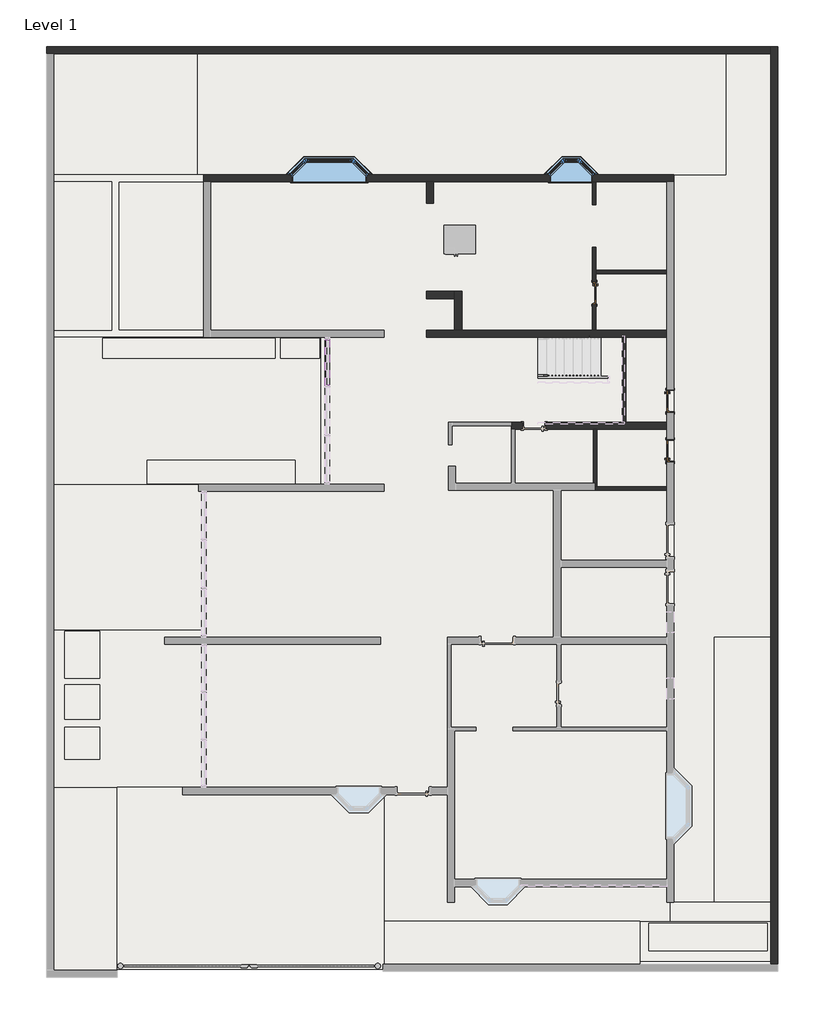
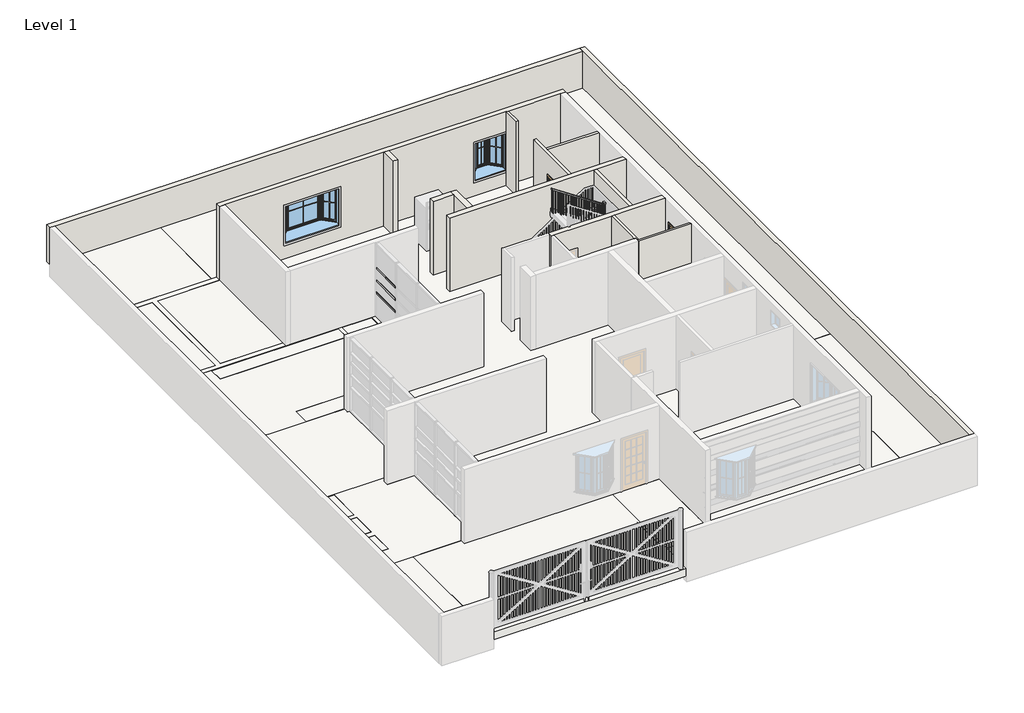
# One storey, part 4 of 5: 15 slabs, 14 walls, 3 doors, 3 members, 2 windows, 1 railing.
"""IFC4 building model written with IfcOpenShell, lengths in millimetres."""

from ifc_helpers import new_model, si_unit, frame, origin, origin_with_axes, place, context, project, spatial, polyline, outline, extrude, faceted_brep, transform, mapped, element, save
from components import door_interior_single_1_panel_wood_5fe0af8f, door_interior_single_1_panel_wood_a1a047a4, door_interior_single_1_panel_wood_33af59b7, member_f9f7e124, window_9f89e8e4, window_bay_casement_45_degree_angle_window_4_787d36ed

model = new_model("IFC4")

# Units and contexts
model_context = context("Model", 3, world=origin())
ifc_project = project(units=[si_unit("LENGTHUNIT", "METRE", prefix="MILLI")], contexts=[model_context])

# Site, building, storey
site = spatial("IfcSite", under=ifc_project)
building = spatial("IfcBuilding", under=site)
storey = spatial("IfcBuildingStorey", under=building, Name="Level 1", Elevation=0.0)

# Doors
placement = place(None, origin())
door_interior_single_1_panel_wood_shape = door_interior_single_1_panel_wood_5fe0af8f(model_context)
element("IfcDoor", 1, ObjectType="Door-Interior-Single-1_Panel-Wood", at=placement, inside=storey, context=model_context, shape_type="MappedRepresentation", body=[
    mapped(door_interior_single_1_panel_wood_shape, transform((-37351.3130314, 2521.1086027, 0.0), x_axis=(0.0, 1.0, 0.0), y_axis=(-1.0, 0.0, 0.0), z_axis=(0.0, 0.0, 1.0))),
])
door_interior_single_1_panel_wood_2_shape = door_interior_single_1_panel_wood_a1a047a4(model_context)
element("IfcDoor", 2, ObjectType="Door-Interior-Single-1_Panel-Wood", at=placement, inside=storey, context=model_context, shape_type="MappedRepresentation", body=[
    mapped(door_interior_single_1_panel_wood_2_shape, transform((-37351.3130314, 3943.5086027, 0.0), x_axis=(0.0, -1.0, 0.0), y_axis=(1.0, 0.0, 0.0), z_axis=(0.0, 0.0, 1.0))),
])
door_interior_single_1_panel_wood_3_shape = door_interior_single_1_panel_wood_33af59b7(model_context)
element("IfcDoor", 3, ObjectType="Door-Interior-Single-1_Panel-Wood", at=placement, inside=storey, context=model_context, shape_type="MappedRepresentation", body=[
    mapped(door_interior_single_1_panel_wood_3_shape, transform((-39529.3630314, 7042.3086027, 0.0), x_axis=(0.0, -1.0, 0.0), y_axis=(1.0, 0.0, 0.0), z_axis=(0.0, 0.0, 1.0))),
])

# Members
member_shape = member_f9f7e124(model_context)
element("IfcMember", 4, ObjectType="Rectangular Mullion : 2.5\" x 5\" rectangular", at=placement, inside=storey, context=model_context, shape_type="MappedRepresentation", body=[
    mapped(member_shape, transform((-47203.3380314, 5708.8086027, 1016.0), x_axis=(0.0, 0.0, 1.0), y_axis=(1.0, 0.0, 0.0), z_axis=(0.0, 1.0, 0.0))),
])
element("IfcMember", 5, ObjectType="Rectangular Mullion : 2.5\" x 5\" rectangular", at=placement, inside=storey, context=model_context, shape_type="MappedRepresentation", body=[
    mapped(member_shape, transform((-47203.3380314, 5708.8086027, 2032.0), x_axis=(0.0, 0.0, 1.0), y_axis=(1.0, 0.0, 0.0), z_axis=(0.0, 1.0, 0.0))),
])
element("IfcMember", 6, ObjectType="Rectangular Mullion : 2.5\" x 5\" rectangular", at=placement, inside=storey, context=model_context, shape_type="MappedRepresentation", body=[
    mapped(member_shape, transform((-47203.3380314, 5708.8086027, 1524.0), x_axis=(0.0, 0.0, 1.0), y_axis=(1.0, 0.0, 0.0), z_axis=(0.0, 1.0, 0.0))),
])

# Railing
element("IfcRailing", 7, ObjectType="Handrail - Rectangular", at=placement, inside=storey, context=model_context, shape_type="SolidModel", body=[
    faceted_brep([(-41148.2472477, 4705.5086027, 1083.7333333), (-41148.2472477, 4705.5086027, 1022.6793317), (-41148.2472477, 4654.7086027, 1022.6793317), (-41148.2472477, 4654.7086027, 1083.7333333), (-39167.0472477, 4705.5086027, 2404.5333333), (-39116.2472477, 4705.5086027, 2377.3459984), (-39116.2472477, 4654.7086027, 2377.3459984), (-39167.0472477, 4654.7086027, 2404.5333333), (-39167.0472477, 4705.5086027, 2438.4), (-39116.2472477, 4705.5086027, 2387.6), (-39116.2472477, 4654.7086027, 2387.6), (-39167.0472477, 4654.7086027, 2438.4), (-39040.0472477, 4705.5086027, 2438.4), (-39040.0472477, 4705.5086027, 2387.6), (-39090.8472477, 4654.7086027, 2387.6), (-39090.8472477, 4654.7086027, 2438.4), (-39040.0472477, 4578.5086027, 2438.4), (-39040.0472477, 4578.5086027, 2387.6), (-39090.8472477, 4578.5086027, 2387.6), (-39090.8472477, 4578.5086027, 2438.4), (-39040.0472477, 4527.7086027, 2438.4), (-39040.0472477, 4476.9086027, 2387.6), (-39090.8472477, 4476.9086027, 2387.6), (-39090.8472477, 4527.7086027, 2438.4), (-39040.0472477, 4527.7086027, 2641.6), (-39040.0472477, 4476.9086027, 2590.8), (-39090.8472477, 4476.9086027, 2590.8), (-39090.8472477, 4527.7086027, 2641.6), (-39040.0472477, 4400.7086027, 2641.6), (-39040.0472477, 4400.7086027, 2590.8), (-39090.8472477, 4451.5086027, 2590.8), (-39090.8472477, 4451.5086027, 2641.6), (-39167.0472477, 4400.7086027, 2641.6), (-39182.4282501, 4400.7086027, 2590.8), (-39182.4282501, 4451.5086027, 2590.8), (-39167.0472477, 4451.5086027, 2641.6), (-41148.2472477, 4400.7086027, 3962.4), (-41148.2472477, 4451.5086027, 3962.4), (-41148.2472477, 4451.5086027, 3901.3459984), (-41148.2472477, 4400.7086027, 3901.3459984)], [[[0, 1, 2, 3]], [[1, 0, 4, 5]], [[2, 1, 5, 6]], [[3, 2, 6, 7]], [[0, 3, 7, 4]], [[5, 4, 8, 9]], [[6, 5, 9, 10]], [[7, 6, 10, 11]], [[4, 7, 11, 8]], [[9, 8, 12, 13]], [[10, 9, 13, 14]], [[11, 10, 14, 15]], [[8, 11, 15, 12]], [[13, 12, 16, 17]], [[14, 13, 17, 18]], [[15, 14, 18, 19]], [[12, 15, 19, 16]], [[17, 16, 20, 21]], [[18, 17, 21, 22]], [[19, 18, 22, 23]], [[16, 19, 23, 20]], [[21, 20, 24, 25]], [[22, 21, 25, 26]], [[23, 22, 26, 27]], [[20, 23, 27, 24]], [[25, 24, 28, 29]], [[26, 25, 29, 30]], [[27, 26, 30, 31]], [[24, 27, 31, 28]], [[29, 28, 32, 33]], [[30, 29, 33, 34]], [[31, 30, 34, 35]], [[28, 31, 35, 32]], [[36, 37, 38, 39]], [[33, 32, 36, 39]], [[34, 33, 39, 38]], [[35, 34, 38, 37]], [[32, 35, 37, 36]]]),
    extrude(outline(polyline([(3861.1293317, -41087.9222477), (3873.8293317, -41106.9722477), (2878.6666667, -41106.9722477), (2878.6666667, -41087.9222477), (3861.1293317, -41087.9222477)])), frame((0.0, 4416.5836027, 0.0), z_axis=(0.0, 1.0, 0.0), x_axis=(0.0, 0.0, 1.0)), (0.0, 0.0, 1.0), 19.05),
    extrude(outline(polyline([(3793.3959984, -40986.3222477), (3806.0959984, -41005.3722477), (2878.6666667, -41005.3722477), (2878.6666667, -40986.3222477), (3793.3959984, -40986.3222477)])), frame((0.0, 4416.5836027, 0.0), z_axis=(0.0, 1.0, 0.0), x_axis=(0.0, 0.0, 1.0)), (0.0, 0.0, 1.0), 19.05),
    extrude(outline(polyline([(3725.6626651, -40884.7222477), (3738.3626651, -40903.7722477), (2878.6666667, -40903.7722477), (2878.6666667, -40884.7222477), (3725.6626651, -40884.7222477)])), frame((0.0, 4416.5836027, 0.0), z_axis=(0.0, 1.0, 0.0), x_axis=(0.0, 0.0, 1.0)), (0.0, 0.0, 1.0), 19.05),
    extrude(outline(polyline([(3657.9293317, -40783.1222477), (3670.6293317, -40802.1722477), (2709.3333333, -40802.1722477), (2709.3333333, -40783.1222477), (3657.9293317, -40783.1222477)])), frame((0.0, 4416.5836027, 0.0), z_axis=(0.0, 1.0, 0.0), x_axis=(0.0, 0.0, 1.0)), (0.0, 0.0, 1.0), 19.05),
    extrude(outline(polyline([(3590.1959984, -40681.5222477), (3602.8959984, -40700.5722477), (2709.3333333, -40700.5722477), (2709.3333333, -40681.5222477), (3590.1959984, -40681.5222477)])), frame((0.0, 4416.5836027, 0.0), z_axis=(0.0, 1.0, 0.0), x_axis=(0.0, 0.0, 1.0)), (0.0, 0.0, 1.0), 19.05),
    extrude(outline(polyline([(3522.4626651, -40579.9222477), (3535.1626651, -40598.9722477), (2540.0, -40598.9722477), (2540.0, -40579.9222477), (3522.4626651, -40579.9222477)])), frame((0.0, 4416.5836027, 0.0), z_axis=(0.0, 1.0, 0.0), x_axis=(0.0, 0.0, 1.0)), (0.0, 0.0, 1.0), 19.05),
    extrude(outline(polyline([(3454.7293317, -40478.3222477), (3467.4293317, -40497.3722477), (2540.0, -40497.3722477), (2540.0, -40478.3222477), (3454.7293317, -40478.3222477)])), frame((0.0, 4416.5836027, 0.0), z_axis=(0.0, 1.0, 0.0), x_axis=(0.0, 0.0, 1.0)), (0.0, 0.0, 1.0), 19.05),
    extrude(outline(polyline([(3386.9959984, -40376.7222477), (3399.6959984, -40395.7722477), (2540.0, -40395.7722477), (2540.0, -40376.7222477), (3386.9959984, -40376.7222477)])), frame((0.0, 4416.5836027, 0.0), z_axis=(0.0, 1.0, 0.0), x_axis=(0.0, 0.0, 1.0)), (0.0, 0.0, 1.0), 19.05),
    extrude(outline(polyline([(3319.2626651, -40275.1222477), (3331.9626651, -40294.1722477), (2370.6666667, -40294.1722477), (2370.6666667, -40275.1222477), (3319.2626651, -40275.1222477)])), frame((0.0, 4416.5836027, 0.0), z_axis=(0.0, 1.0, 0.0), x_axis=(0.0, 0.0, 1.0)), (0.0, 0.0, 1.0), 19.05),
    extrude(outline(polyline([(3251.5293317, -40173.5222477), (3264.2293317, -40192.5722477), (2370.6666667, -40192.5722477), (2370.6666667, -40173.5222477), (3251.5293317, -40173.5222477)])), frame((0.0, 4416.5836027, 0.0), z_axis=(0.0, 1.0, 0.0), x_axis=(0.0, 0.0, 1.0)), (0.0, 0.0, 1.0), 19.05),
    extrude(outline(polyline([(3183.7959984, -40071.9222477), (3196.4959984, -40090.9722477), (2201.3333333, -40090.9722477), (2201.3333333, -40071.9222477), (3183.7959984, -40071.9222477)])), frame((0.0, 4416.5836027, 0.0), z_axis=(0.0, 1.0, 0.0), x_axis=(0.0, 0.0, 1.0)), (0.0, 0.0, 1.0), 19.05),
    extrude(outline(polyline([(3116.0626651, -39970.3222477), (3128.7626651, -39989.3722477), (2201.3333333, -39989.3722477), (2201.3333333, -39970.3222477), (3116.0626651, -39970.3222477)])), frame((0.0, 4416.5836027, 0.0), z_axis=(0.0, 1.0, 0.0), x_axis=(0.0, 0.0, 1.0)), (0.0, 0.0, 1.0), 19.05),
    extrude(outline(polyline([(3048.3293317, -39868.7222477), (3061.0293317, -39887.7722477), (2201.3333333, -39887.7722477), (2201.3333333, -39868.7222477), (3048.3293317, -39868.7222477)])), frame((0.0, 4416.5836027, 0.0), z_axis=(0.0, 1.0, 0.0), x_axis=(0.0, 0.0, 1.0)), (0.0, 0.0, 1.0), 19.05),
    extrude(outline(polyline([(2980.5959984, -39767.1222477), (2993.2959984, -39786.1722477), (2032.0, -39786.1722477), (2032.0, -39767.1222477), (2980.5959984, -39767.1222477)])), frame((0.0, 4416.5836027, 0.0), z_axis=(0.0, 1.0, 0.0), x_axis=(0.0, 0.0, 1.0)), (0.0, 0.0, 1.0), 19.05),
    extrude(outline(polyline([(2912.8626651, -39665.5222477), (2925.5626651, -39684.5722477), (2032.0, -39684.5722477), (2032.0, -39665.5222477), (2912.8626651, -39665.5222477)])), frame((0.0, 4416.5836027, 0.0), z_axis=(0.0, 1.0, 0.0), x_axis=(0.0, 0.0, 1.0)), (0.0, 0.0, 1.0), 19.05),
    extrude(outline(polyline([(2845.1293317, -39563.9222477), (2857.8293317, -39582.9722477), (1862.6666667, -39582.9722477), (1862.6666667, -39563.9222477), (2845.1293317, -39563.9222477)])), frame((0.0, 4416.5836027, 0.0), z_axis=(0.0, 1.0, 0.0), x_axis=(0.0, 0.0, 1.0)), (0.0, 0.0, 1.0), 19.05),
    extrude(outline(polyline([(2777.3959984, -39462.3222477), (2790.0959984, -39481.3722477), (1862.6666667, -39481.3722477), (1862.6666667, -39462.3222477), (2777.3959984, -39462.3222477)])), frame((0.0, 4416.5836027, 0.0), z_axis=(0.0, 1.0, 0.0), x_axis=(0.0, 0.0, 1.0)), (0.0, 0.0, 1.0), 19.05),
    extrude(outline(polyline([(2709.6626651, -39360.7222477), (2722.3626651, -39379.7722477), (1862.6666667, -39379.7722477), (1862.6666667, -39360.7222477), (2709.6626651, -39360.7222477)])), frame((0.0, 4416.5836027, 0.0), z_axis=(0.0, 1.0, 0.0), x_axis=(0.0, 0.0, 1.0)), (0.0, 0.0, 1.0), 19.05),
    extrude(outline(polyline([(2641.9293317, -39259.1222477), (2654.6293317, -39278.1722477), (1693.3333333, -39278.1722477), (1693.3333333, -39259.1222477), (2641.9293317, -39259.1222477)])), frame((0.0, 4416.5836027, 0.0), z_axis=(0.0, 1.0, 0.0), x_axis=(0.0, 0.0, 1.0)), (0.0, 0.0, 1.0), 19.05),
    extrude(outline(polyline([(2574.1959984, -39157.5222477), (2586.8959984, -39176.5722477), (1693.3333333, -39176.5722477), (1693.3333333, -39157.5222477), (2574.1959984, -39157.5222477)])), frame((0.0, 4416.5836027, 0.0), z_axis=(0.0, 1.0, 0.0), x_axis=(0.0, 0.0, 1.0)), (0.0, 0.0, 1.0), 19.05),
    extrude(outline(polyline([(-39074.9722477, 4486.4336027), (-39055.9222477, 4486.4336027), (-39055.9222477, 4467.3836027), (-39074.9722477, 4467.3836027), (-39074.9722477, 4486.4336027)])), frame((0.0, 0.0, 1524.0), z_axis=(0.0, 0.0, 1.0), x_axis=(1.0, 0.0, 0.0)), (0.0, 0.0, 1.0), 1066.8),
    extrude(outline(polyline([(-39074.9722477, 4588.0336027), (-39055.9222477, 4588.0336027), (-39055.9222477, 4568.9836027), (-39074.9722477, 4568.9836027), (-39074.9722477, 4588.0336027)])), frame((0.0, 0.0, 1524.0), z_axis=(0.0, 0.0, 1.0), x_axis=(1.0, 0.0, 0.0)), (0.0, 0.0, 1.0), 863.6),
    extrude(outline(polyline([(-39125.7722477, 4670.5836027), (-39125.7722477, 4689.6336027), (-39106.7222477, 4689.6336027), (-39106.7222477, 4670.5836027), (-39125.7722477, 4670.5836027)])), frame((0.0, 0.0, 1524.0), z_axis=(0.0, 0.0, 1.0), x_axis=(1.0, 0.0, 0.0)), (0.0, 0.0, 1.0), 863.6),
    extrude(outline(polyline([(2315.9626651, -39208.3222477), (2303.2626651, -39227.3722477), (1354.6666667, -39227.3722477), (1354.6666667, -39208.3222477), (2315.9626651, -39208.3222477)])), frame((0.0, 4670.5836027, 0.0), z_axis=(0.0, 1.0, 0.0), x_axis=(0.0, 0.0, 1.0)), (0.0, 0.0, 1.0), 19.05),
    extrude(outline(polyline([(2248.2293317, -39309.9222477), (2235.5293317, -39328.9722477), (1354.6666667, -39328.9722477), (1354.6666667, -39309.9222477), (2248.2293317, -39309.9222477)])), frame((0.0, 4670.5836027, 0.0), z_axis=(0.0, 1.0, 0.0), x_axis=(0.0, 0.0, 1.0)), (0.0, 0.0, 1.0), 19.05),
    extrude(outline(polyline([(2180.4959984, -39411.5222477), (2167.7959984, -39430.5722477), (1185.3333333, -39430.5722477), (1185.3333333, -39411.5222477), (2180.4959984, -39411.5222477)])), frame((0.0, 4670.5836027, 0.0), z_axis=(0.0, 1.0, 0.0), x_axis=(0.0, 0.0, 1.0)), (0.0, 0.0, 1.0), 19.05),
    extrude(outline(polyline([(2112.7626651, -39513.1222477), (2100.0626651, -39532.1722477), (1185.3333333, -39532.1722477), (1185.3333333, -39513.1222477), (2112.7626651, -39513.1222477)])), frame((0.0, 4670.5836027, 0.0), z_axis=(0.0, 1.0, 0.0), x_axis=(0.0, 0.0, 1.0)), (0.0, 0.0, 1.0), 19.05),
    extrude(outline(polyline([(2045.0293317, -39614.7222477), (2032.3293317, -39633.7722477), (1185.3333333, -39633.7722477), (1185.3333333, -39614.7222477), (2045.0293317, -39614.7222477)])), frame((0.0, 4670.5836027, 0.0), z_axis=(0.0, 1.0, 0.0), x_axis=(0.0, 0.0, 1.0)), (0.0, 0.0, 1.0), 19.05),
    extrude(outline(polyline([(1977.2959984, -39716.3222477), (1964.5959984, -39735.3722477), (1016.0, -39735.3722477), (1016.0, -39716.3222477), (1977.2959984, -39716.3222477)])), frame((0.0, 4670.5836027, 0.0), z_axis=(0.0, 1.0, 0.0), x_axis=(0.0, 0.0, 1.0)), (0.0, 0.0, 1.0), 19.05),
    extrude(outline(polyline([(1909.5626651, -39817.9222477), (1896.8626651, -39836.9722477), (1016.0, -39836.9722477), (1016.0, -39817.9222477), (1909.5626651, -39817.9222477)])), frame((0.0, 4670.5836027, 0.0), z_axis=(0.0, 1.0, 0.0), x_axis=(0.0, 0.0, 1.0)), (0.0, 0.0, 1.0), 19.05),
    extrude(outline(polyline([(1841.8293317, -39919.5222477), (1829.1293317, -39938.5722477), (846.6666667, -39938.5722477), (846.6666667, -39919.5222477), (1841.8293317, -39919.5222477)])), frame((0.0, 4670.5836027, 0.0), z_axis=(0.0, 1.0, 0.0), x_axis=(0.0, 0.0, 1.0)), (0.0, 0.0, 1.0), 19.05),
    extrude(outline(polyline([(1774.0959984, -40021.1222477), (1761.3959984, -40040.1722477), (846.6666667, -40040.1722477), (846.6666667, -40021.1222477), (1774.0959984, -40021.1222477)])), frame((0.0, 4670.5836027, 0.0), z_axis=(0.0, 1.0, 0.0), x_axis=(0.0, 0.0, 1.0)), (0.0, 0.0, 1.0), 19.05),
    extrude(outline(polyline([(1706.3626651, -40122.7222477), (1693.6626651, -40141.7722477), (846.6666667, -40141.7722477), (846.6666667, -40122.7222477), (1706.3626651, -40122.7222477)])), frame((0.0, 4670.5836027, 0.0), z_axis=(0.0, 1.0, 0.0), x_axis=(0.0, 0.0, 1.0)), (0.0, 0.0, 1.0), 19.05),
    extrude(outline(polyline([(1638.6293317, -40224.3222477), (1625.9293317, -40243.3722477), (677.3333333, -40243.3722477), (677.3333333, -40224.3222477), (1638.6293317, -40224.3222477)])), frame((0.0, 4670.5836027, 0.0), z_axis=(0.0, 1.0, 0.0), x_axis=(0.0, 0.0, 1.0)), (0.0, 0.0, 1.0), 19.05),
    extrude(outline(polyline([(1570.8959984, -40325.9222477), (1558.1959984, -40344.9722477), (677.3333333, -40344.9722477), (677.3333333, -40325.9222477), (1570.8959984, -40325.9222477)])), frame((0.0, 4670.5836027, 0.0), z_axis=(0.0, 1.0, 0.0), x_axis=(0.0, 0.0, 1.0)), (0.0, 0.0, 1.0), 19.05),
    extrude(outline(polyline([(1503.1626651, -40427.5222477), (1490.4626651, -40446.5722477), (508.0, -40446.5722477), (508.0, -40427.5222477), (1503.1626651, -40427.5222477)])), frame((0.0, 4670.5836027, 0.0), z_axis=(0.0, 1.0, 0.0), x_axis=(0.0, 0.0, 1.0)), (0.0, 0.0, 1.0), 19.05),
    extrude(outline(polyline([(1435.4293317, -40529.1222477), (1422.7293317, -40548.1722477), (508.0, -40548.1722477), (508.0, -40529.1222477), (1435.4293317, -40529.1222477)])), frame((0.0, 4670.5836027, 0.0), z_axis=(0.0, 1.0, 0.0), x_axis=(0.0, 0.0, 1.0)), (0.0, 0.0, 1.0), 19.05),
    extrude(outline(polyline([(1367.6959984, -40630.7222477), (1354.9959984, -40649.7722477), (508.0, -40649.7722477), (508.0, -40630.7222477), (1367.6959984, -40630.7222477)])), frame((0.0, 4670.5836027, 0.0), z_axis=(0.0, 1.0, 0.0), x_axis=(0.0, 0.0, 1.0)), (0.0, 0.0, 1.0), 19.05),
    extrude(outline(polyline([(1299.9626651, -40732.3222477), (1287.2626651, -40751.3722477), (338.6666667, -40751.3722477), (338.6666667, -40732.3222477), (1299.9626651, -40732.3222477)])), frame((0.0, 4670.5836027, 0.0), z_axis=(0.0, 1.0, 0.0), x_axis=(0.0, 0.0, 1.0)), (0.0, 0.0, 1.0), 19.05),
    extrude(outline(polyline([(1232.2293317, -40833.9222477), (1219.5293317, -40852.9722477), (338.6666667, -40852.9722477), (338.6666667, -40833.9222477), (1232.2293317, -40833.9222477)])), frame((0.0, 4670.5836027, 0.0), z_axis=(0.0, 1.0, 0.0), x_axis=(0.0, 0.0, 1.0)), (0.0, 0.0, 1.0), 19.05),
    extrude(outline(polyline([(1164.4959984, -40935.5222477), (1151.7959984, -40954.5722477), (169.3333333, -40954.5722477), (169.3333333, -40935.5222477), (1164.4959984, -40935.5222477)])), frame((0.0, 4670.5836027, 0.0), z_axis=(0.0, 1.0, 0.0), x_axis=(0.0, 0.0, 1.0)), (0.0, 0.0, 1.0), 19.05),
    extrude(outline(polyline([(1096.7626651, -41037.1222477), (1084.0626651, -41056.1722477), (169.3333333, -41056.1722477), (169.3333333, -41037.1222477), (1096.7626651, -41037.1222477)])), frame((0.0, 4670.5836027, 0.0), z_axis=(0.0, 1.0, 0.0), x_axis=(0.0, 0.0, 1.0)), (0.0, 0.0, 1.0), 19.05),
    extrude(outline(polyline([(-39074.9722477, 4435.6336027), (-39055.9222477, 4435.6336027), (-39055.9222477, 4416.5836027), (-39074.9722477, 4416.5836027), (-39074.9722477, 4435.6336027)])), frame((0.0, 0.0, 1524.0), z_axis=(0.0, 0.0, 1.0), x_axis=(1.0, 0.0, 0.0)), (0.0, 0.0, 1.0), 1066.8),
    extrude(outline(polyline([(-39074.9722477, 4670.5836027), (-39074.9722477, 4689.6336027), (-39055.9222477, 4689.6336027), (-39055.9222477, 4670.5836027), (-39074.9722477, 4670.5836027)])), frame((0.0, 0.0, 1524.0), z_axis=(0.0, 0.0, 1.0), x_axis=(1.0, 0.0, 0.0)), (0.0, 0.0, 1.0), 863.6),
    extrude(outline(polyline([(3888.6459984, -41129.1972477), (3901.3459984, -41148.2472477), (2878.6666667, -41148.2472477), (2878.6666667, -41129.1972477), (3888.6459984, -41129.1972477)])), frame((0.0, 4416.5836027, 0.0), z_axis=(0.0, 1.0, 0.0), x_axis=(0.0, 0.0, 1.0)), (0.0, 0.0, 1.0), 19.05),
    extrude(outline(polyline([(1035.3793317, -41129.1972477), (1022.6793317, -41148.2472477), (169.3333333, -41148.2472477), (169.3333333, -41129.1972477), (1035.3793317, -41129.1972477)])), frame((0.0, 4670.5836027, 0.0), z_axis=(0.0, 1.0, 0.0), x_axis=(0.0, 0.0, 1.0)), (0.0, 0.0, 1.0), 19.05),
])

# Slabs
element("IfcSlab", 8, at=placement, inside=storey, context=model_context, shape_type="SweptSolid", body=[
    extrude(outline(polyline([(-50956.4260686, 13968.3227856), (-50956.4260686, 10445.9086027), (-55177.8412112, 10445.9086027), (-55177.8412112, 13968.3227856), (-50956.4260686, 13968.3227856)])), frame((0.0, 0.0, -304.8), z_axis=(0.0, 0.0, 1.0), x_axis=(1.0, 0.0, 0.0)), (0.0, 0.0, 1.0), 304.8),
    extrude(outline(polyline([(-38223.6402545, -12148.7888585), (-38223.6402545, -11006.389557), (-34350.9380314, -11006.389557), (-34350.9380314, -12148.7888585), (-38223.6402545, -12148.7888585)]), holes=[polyline([(-37969.6402545, -11843.9888585), (-34554.1380314, -11843.9888585), (-34554.1380314, -11057.189557), (-37969.6402545, -11057.189557), (-37969.6402545, -11843.9888585)])]), frame((0.0, 0.0, -304.8), z_axis=(0.0, 0.0, 1.0), x_axis=(1.0, 0.0, 0.0)), (0.0, 0.0, 1.0), 304.8),
])
element("IfcSlab", 9, at=placement, inside=storey, context=model_context, shape_type="SweptSolid", body=[
    extrude(outline(polyline([(-34350.9380314, -2838.2913973), (-34350.9380314, -10458.2913973), (-36081.491084, -10458.2913973), (-36081.491084, -2838.2913973), (-34350.9380314, -2838.2913973)])), frame((0.0, 0.0, -304.8), z_axis=(0.0, 0.0, 1.0), x_axis=(1.0, 0.0, 0.0)), (0.0, 0.0, 1.0), 304.8),
])
element("IfcSlab", 10, at=placement, inside=storey, context=model_context, shape_type="SweptSolid", body=[
    extrude(outline(polyline([(-55177.8412112, 10445.9086027), (-50759.3380314, 10445.9086027), (-50759.3380314, 10242.7086027), (-53197.7380314, 10242.7086027), (-53197.7380314, 5975.5086027), (-50759.3380314, 5975.5086027), (-50759.3380314, 5772.3086027), (-55204.3380314, 5772.3086027), (-55204.3380314, 5975.5086027), (-53400.9380314, 5975.5086027), (-53400.9380314, 10242.7086027), (-55204.3380314, 10242.7086027), (-55204.3380314, 10445.9086027), (-55177.8412112, 10445.9086027)])), frame((0.0, 0.0, -304.8), z_axis=(0.0, 0.0, 1.0), x_axis=(1.0, 0.0, 0.0)), (0.0, 0.0, 1.0), 304.8),
])
element("IfcSlab", 11, ObjectType="GRASS TYPE 1'", at=placement, inside=storey, context=model_context, shape_type="SweptSolid", body=[
    extrude(outline(polyline([(-55204.3380314, -2635.0913973), (-50759.3380314, -2635.0913973), (-50759.3380314, -7156.2913973), (-55204.3380314, -7156.2913973), (-55204.3380314, -2635.0913973)]), holes=[polyline([(-53746.793915, -4017.7088102), (-53746.793915, -2671.5088102), (-54750.550784, -2671.5088102), (-54750.550784, -4017.7088102), (-53746.793915, -4017.7088102)]), polyline([(-54750.550784, -4205.0162107), (-54750.550784, -5196.8737449), (-53746.793915, -5196.8737449), (-53746.793915, -4205.0162107), (-54750.550784, -4205.0162107)]), polyline([(-54750.550784, -5426.5355358), (-54750.550784, -6340.9585066), (-53746.793915, -6340.9585066), (-53746.793915, -5426.5355358), (-54750.550784, -5426.5355358)])]), frame((0.0, 0.0, -304.8), z_axis=(0.0, 0.0, 1.0), x_axis=(1.0, 0.0, 0.0)), (0.0, 0.0, 1.0), 304.8),
])
element("IfcSlab", 12, ObjectType="GRASS TYPE 1'", at=placement, inside=storey, context=model_context, shape_type="SweptSolid", body=[
    extrude(outline(polyline([(-55204.3380314, 5772.3086027), (-47406.5380314, 5772.3086027), (-47406.5380314, 1555.9086027), (-55204.3380314, 1555.9086027), (-55204.3380314, 5772.3086027)]), holes=[polyline([(-48135.4981877, 2238.2630791), (-52386.7116594, 2238.2630791), (-52386.7116594, 1573.668759), (-48135.4981877, 1573.668759), (-48135.4981877, 2238.2630791)]), polyline([(-47424.2981877, 5180.468759), (-47424.2981877, 5754.5484465), (-48553.7407394, 5754.5484465), (-48553.7407394, 5180.468759), (-47424.2981877, 5180.468759)]), polyline([(-48713.9410385, 5180.468759), (-48713.9410385, 5754.5484465), (-53668.2114737, 5754.5484465), (-53668.2114737, 5180.468759), (-48713.9410385, 5180.468759)])]), frame((0.0, 0.0, -304.8), z_axis=(0.0, 0.0, 1.0), x_axis=(1.0, 0.0, 0.0)), (0.0, 0.0, 1.0), 304.8),
])
element("IfcSlab", 13, ObjectType="GRASS TYPE 1'", at=placement, inside=storey, context=model_context, shape_type="SweptSolid", body=[
    extrude(outline(polyline([(-55204.3380314, -7156.2913973), (-53248.5380314, -7156.2913973), (-53248.5380314, -12388.6913973), (-55204.3380314, -12388.6913973), (-55204.3380314, -7156.2913973)])), frame((0.0, 0.0, -304.8), z_axis=(0.0, 0.0, 1.0), x_axis=(1.0, 0.0, 0.0)), (0.0, 0.0, 1.0), 304.8),
    extrude(outline(polyline([(-45577.7380314, -11006.389557), (-38223.6402545, -11006.389557), (-38223.6402545, -12386.9889249), (-45577.7380314, -12386.9889249), (-45577.7380314, -11006.389557)])), frame((0.0, 0.0, -304.8), z_axis=(0.0, 0.0, 1.0), x_axis=(1.0, 0.0, 0.0)), (0.0, 0.0, 1.0), 304.8),
    extrude(outline(polyline([(-37969.6402545, -11057.189557), (-34554.1380314, -11057.189557), (-34554.1380314, -11843.9888585), (-37969.6402545, -11843.9888585), (-37969.6402545, -11057.189557)])), frame((0.0, 0.0, -304.8), z_axis=(0.0, 0.0, 1.0), x_axis=(1.0, 0.0, 0.0)), (0.0, 0.0, 1.0), 304.8),
])
element("IfcSlab", 14, ObjectType="GRASS TYPE 1'", at=placement, inside=storey, context=model_context, shape_type="SweptSolid", body=[
    extrude(outline(polyline([(-50759.3380314, 10242.7086027), (-50759.3380314, 5975.5086027), (-53197.7380314, 5975.5086027), (-53197.7380314, 10242.7086027), (-50759.3380314, 10242.7086027)])), frame((0.0, 0.0, -304.8), z_axis=(0.0, 0.0, 1.0), x_axis=(1.0, 0.0, 0.0)), (0.0, 0.0, 1.0), 304.8),
])
element("IfcSlab", 15, ObjectType="LW Concrete on Metal Deck", at=placement, inside=storey, context=model_context, shape_type="SweptSolid", body=[
    extrude(outline(polyline([(-34350.9380314, -10458.2913973), (-34350.9380314, -11006.389557), (-37360.0402545, -11006.389557), (-37360.0402545, -10458.2913973), (-34350.9380314, -10458.2913973)])), frame((0.0, 0.0, -104.775), z_axis=(0.0, 0.0, 1.0), x_axis=(1.0, 0.0, 0.0)), (0.0, 0.0, 1.0), 104.775),
])
element("IfcSlab", 16, ObjectType="MARBLE FLOORING 1'", at=placement, inside=storey, context=model_context, shape_type="SweptSolid", body=[
    extrude(outline(polyline([(-37246.5380314, 10445.9086027), (-37246.5380314, -10001.0913973), (-43748.9380314, -10001.0913973), (-43748.9380314, -7359.4913973), (-51368.9380314, -7359.4913973), (-51368.9380314, -7156.2913973), (-50759.3380314, -7156.2913973), (-50759.3380314, -3041.4913973), (-51880.9582963, -3041.4913973), (-51880.9582963, -2838.2913973), (-50759.3380314, -2838.2913973), (-50759.3380314, 1555.9086027), (-47406.5380314, 1555.9086027), (-47406.5380314, 5772.3086027), (-50759.3380314, 5772.3086027), (-50759.3380314, 10445.9086027), (-37246.5380314, 10445.9086027)])), frame((0.0, 0.0, -304.8), z_axis=(0.0, 0.0, 1.0), x_axis=(1.0, 0.0, 0.0)), (0.0, 0.0, 1.0), 304.8),
])
element("IfcSlab", 17, ObjectType="MARBLE FLOORING 1' 2", at=placement, inside=storey, context=model_context, shape_type="SweptSolid", body=[
    extrude(outline(polyline([(-45577.7380314, -7156.2913973), (-45577.7380314, -12386.9889249), (-53248.5380314, -12386.9889249), (-53248.5380314, -7156.2913973), (-45577.7380314, -7156.2913973)])), frame((0.0, 0.0, -304.8), z_axis=(0.0, 0.0, 1.0), x_axis=(1.0, 0.0, 0.0)), (0.0, 0.0, 1.0), 304.8),
])
element("IfcSlab", 18, ObjectType="VERANDA FLOORING 1'", at=placement, inside=storey, context=model_context, shape_type="SweptSolid", body=[
    extrude(outline(polyline([(-35747.9380314, 10445.9086027), (-35747.9380314, 13951.1086027), (-34350.9380314, 13951.1086027), (-34350.9380314, 10445.9086027), (-34350.9380314, -2838.2913973), (-36081.491084, -2838.2913973), (-36081.491084, -10458.2913973), (-37246.5380314, -10458.2913973), (-37246.5380314, 10445.9086027), (-35747.9380314, 10445.9086027)])), frame((0.0, 0.0, -304.8), z_axis=(0.0, 0.0, 1.0), x_axis=(1.0, 0.0, 0.0)), (0.0, 0.0, 1.0), 304.8),
])
element("IfcSlab", 19, ObjectType="VERANDA FLOORING 1'", at=placement, inside=storey, context=model_context, shape_type="SweptSolid", body=[
    extrude(outline(polyline([(-37360.0402545, -11006.389557), (-45577.7380314, -11006.389557), (-45679.3380314, -11006.389557), (-45679.3380314, -7359.4913973), (-43748.9380314, -7359.4913973), (-43748.9380314, -10001.0913973), (-37449.7380314, -10001.0913973), (-37360.0402545, -10001.0913973), (-37360.0402545, -11006.389557)])), frame((0.0, 0.0, -304.8), z_axis=(0.0, 0.0, 1.0), x_axis=(1.0, 0.0, 0.0)), (0.0, 0.0, 1.0), 304.8),
])
element("IfcSlab", 20, ObjectType="VERANDA FLOORING 1'", at=placement, inside=storey, context=model_context, shape_type="SweptSolid", body=[
    extrude(outline(polyline([(-48553.7407394, 5754.5484465), (-47424.2981877, 5754.5484465), (-47424.2981877, 5180.468759), (-48553.7407394, 5180.468759), (-48553.7407394, 5754.5484465)])), frame((0.0, 0.0, -304.8), z_axis=(0.0, 0.0, 1.0), x_axis=(1.0, 0.0, 0.0)), (0.0, 0.0, 1.0), 304.8),
    extrude(outline(polyline([(-53668.2114737, 5754.5484465), (-48713.9410385, 5754.5484465), (-48713.9410385, 5180.468759), (-53668.2114737, 5180.468759), (-53668.2114737, 5754.5484465)])), frame((0.0, 0.0, -304.8), z_axis=(0.0, 0.0, 1.0), x_axis=(1.0, 0.0, 0.0)), (0.0, 0.0, 1.0), 304.8),
    extrude(outline(polyline([(-52386.7116594, 2238.2630791), (-48135.4981877, 2238.2630791), (-48135.4981877, 1573.668759), (-52386.7116594, 1573.668759), (-52386.7116594, 2238.2630791)])), frame((0.0, 0.0, -304.8), z_axis=(0.0, 0.0, 1.0), x_axis=(1.0, 0.0, 0.0)), (0.0, 0.0, 1.0), 304.8),
    extrude(outline(polyline([(-54750.550784, -2671.5088102), (-53746.793915, -2671.5088102), (-53746.793915, -4017.7088102), (-54750.550784, -4017.7088102), (-54750.550784, -2671.5088102)])), frame((0.0, 0.0, -304.8), z_axis=(0.0, 0.0, 1.0), x_axis=(1.0, 0.0, 0.0)), (0.0, 0.0, 1.0), 304.8),
    extrude(outline(polyline([(-54750.550784, -4205.0162107), (-53746.793915, -4205.0162107), (-53746.793915, -5196.8737449), (-54750.550784, -5196.8737449), (-54750.550784, -4205.0162107)])), frame((0.0, 0.0, -304.8), z_axis=(0.0, 0.0, 1.0), x_axis=(1.0, 0.0, 0.0)), (0.0, 0.0, 1.0), 304.8),
    extrude(outline(polyline([(-54750.550784, -5426.5355358), (-53746.793915, -5426.5355358), (-53746.793915, -6340.9585066), (-54750.550784, -6340.9585066), (-54750.550784, -5426.5355358)])), frame((0.0, 0.0, -304.8), z_axis=(0.0, 0.0, 1.0), x_axis=(1.0, 0.0, 0.0)), (0.0, 0.0, 1.0), 304.8),
])
element("IfcSlab", 21, ObjectType="WATER BODY 1'", at=placement, inside=storey, context=model_context, shape_type="SweptSolid", body=[
    extrude(outline(polyline([(-53400.9380314, 10242.7086027), (-53400.9380314, 5975.5086027), (-55204.3380314, 5975.5086027), (-55204.3380314, 10242.7086027), (-53400.9380314, 10242.7086027)])), frame((0.0, 0.0, -304.8), z_axis=(0.0, 0.0, 1.0), x_axis=(1.0, 0.0, 0.0)), (0.0, 0.0, 1.0), 304.8),
])
element("IfcSlab", 22, ObjectType="WOOD DECK 1'", at=placement, inside=storey, context=model_context, shape_type="SweptSolid", body=[
    extrude(outline(polyline([(-50759.3380314, 1555.9086027), (-50759.3380314, -2635.0913973), (-55204.3380314, -2635.0913973), (-55204.3380314, 1555.9086027), (-50759.3380314, 1555.9086027)])), frame((0.0, 0.0, -304.8), z_axis=(0.0, 0.0, 1.0), x_axis=(1.0, 0.0, 0.0)), (0.0, 0.0, 1.0), 304.8),
    extrude(outline(polyline([(-35747.9380314, 13951.1086027), (-35747.9380314, 10445.9086027), (-50956.4260686, 10445.9086027), (-50956.4260686, 13951.1086027), (-35747.9380314, 13951.1086027)])), frame((0.0, 0.0, -304.8), z_axis=(0.0, 0.0, 1.0), x_axis=(1.0, 0.0, 0.0)), (0.0, 0.0, 1.0), 304.8),
])

# Walls
element("IfcWall", 23, ObjectType="INNER WALL 4\"", at=placement, inside=storey, context=model_context, shape_type="Brep", body=[
    faceted_brep([(-37449.7380314, 1479.7086027, 0.0), (-39456.3380314, 1479.7086027, 0.0), (-39507.1380314, 1479.7086027, 0.0), (-39507.1380314, 1479.7086027, 3048.0), (-39456.3380314, 1479.7086027, 3048.0), (-37449.7380314, 1479.7086027, 3048.0), (-37449.7380314, 1378.1086027, 0.0), (-37449.7380314, 1378.1086027, 3048.0), (-39507.1380314, 1378.1086027, 3048.0), (-39507.1380314, 1378.1086027, 0.0)], [[[0, 1, 2, 3, 4, 5]], [[6, 7, 8, 9]], [[2, 1, 0, 6, 9]], [[3, 2, 9, 8]], [[5, 4, 3, 8, 7]], [[0, 5, 7, 6]]]),
])
element("IfcWall", 24, ObjectType="INNER WALL 4\"", at=placement, inside=storey, context=model_context, shape_type="SweptSolid", body=[
    extrude(outline(polyline([(-39557.9380314, 1581.3086027), (-39557.9380314, 3130.7086027), (-39456.3380314, 3130.7086027), (-39456.3380314, 1479.7086027), (-39507.1380314, 1479.7086027), (-39507.1380314, 1581.3086027), (-39557.9380314, 1581.3086027)])), origin_with_axes(), (0.0, 0.0, 1.0), 3048.0),
])
element("IfcWall", 25, ObjectType="INNER WALL 4\"", at=placement, inside=storey, context=model_context, shape_type="SweptSolid", body=[
    extrude(outline(polyline([(-38618.1380314, 5772.3086027), (-38618.1380314, 3333.9086027), (-38719.7380314, 3333.9086027), (-38719.7380314, 5772.3086027), (-38618.1380314, 5772.3086027)])), origin_with_axes(), (0.0, 0.0, 1.0), 3048.0),
])
element("IfcWall", 26, ObjectType="INNER WALL 4\"", at=placement, inside=storey, context=model_context, shape_type="Brep", body=[
    faceted_brep([(-39481.7380314, 8363.1086027, 0.0), (-39481.7380314, 8363.1086027, 3048.0), (-39481.7380314, 7702.7086027, 3048.0), (-39481.7380314, 7601.1086027, 3048.0), (-39481.7380314, 5975.5086027, 3048.0), (-39481.7380314, 5975.5086027, 0.0), (-39481.7380314, 6712.1086027, 0.0), (-39481.7380314, 6712.1086027, 2159.0), (-39481.7380314, 7372.5086027, 2159.0), (-39481.7380314, 7372.5086027, 0.0), (-39481.7380314, 7601.1086027, 0.0), (-39481.7380314, 7702.7086027, 0.0), (-39583.3380314, 8363.1086027, 3048.0), (-39583.3380314, 8363.1086027, 0.0), (-39583.3380314, 7372.5086027, 0.0), (-39583.3380314, 7372.5086027, 2159.0), (-39583.3380314, 6712.1086027, 2159.0), (-39583.3380314, 6712.1086027, 0.0), (-39583.3380314, 5975.5086027, 0.0), (-39583.3380314, 5975.5086027, 3048.0)], [[[0, 1, 2, 3, 4, 5, 6, 7, 8, 9, 10, 11]], [[12, 13, 14, 15, 16, 17, 18, 19]], [[13, 0, 11, 10, 9, 14]], [[5, 18, 17, 6]], [[1, 0, 13, 12]], [[4, 3, 2, 1, 12, 19]], [[5, 4, 19, 18]], [[16, 7, 6, 17]], [[7, 16, 15, 8]], [[8, 15, 14, 9]]]),
])
element("IfcWall", 27, ObjectType="INNER WALL 4\"", at=placement, inside=storey, context=model_context, shape_type="SweptSolid", body=[
    extrude(outline(polyline([(-39481.7380314, 7702.7086027), (-37449.7380314, 7702.7086027), (-37449.7380314, 7601.1086027), (-39481.7380314, 7601.1086027), (-39481.7380314, 7702.7086027)])), origin_with_axes(), (0.0, 0.0, 1.0), 3048.0),
])
element("IfcWall", 28, ObjectType="INNER WALL 4\"", at=placement, inside=storey, context=model_context, shape_type="SweptSolid", body=[
    extrude(outline(polyline([(-39481.7380314, 10242.7086027), (-39481.7380314, 9582.3086027), (-39583.3380314, 9582.3086027), (-39583.3380314, 10242.7086027), (-39481.7380314, 10242.7086027)])), origin_with_axes(), (0.0, 0.0, 1.0), 3048.0),
])
element("IfcWall", 29, ObjectType="OUTER WALL 8\"", at=placement, inside=storey, context=model_context, shape_type="Brep", body=[
    faceted_brep([(-37246.5380314, 10445.9086027, 0.0), (-50759.3380314, 10445.9086027, 0.0), (-50759.3380314, 10445.9086027, 3048.0), (-37246.5380314, 10445.9086027, 3048.0), (-46036.3466227, 10445.9086027, 2184.4), (-48268.7294401, 10445.9086027, 2184.4), (-48268.7294401, 10445.9086027, 609.6), (-46036.3466227, 10445.9086027, 609.6), (-39533.9466227, 10445.9086027, 2184.4), (-40851.9294401, 10445.9086027, 2184.4), (-40851.9294401, 10445.9086027, 609.6), (-39533.9466227, 10445.9086027, 609.6), (-37246.5380314, 10242.7086027, 0.0), (-37246.5380314, 10242.7086027, 3048.0), (-37449.7380314, 10242.7086027, 3048.0), (-39481.7380314, 10242.7086027, 3048.0), (-39583.3380314, 10242.7086027, 3048.0), (-44155.3380314, 10242.7086027, 3048.0), (-44358.5380314, 10242.7086027, 3048.0), (-50556.1380314, 10242.7086027, 3048.0), (-50759.3380314, 10242.7086027, 3048.0), (-50759.3380314, 10242.7086027, 0.0), (-50556.1380314, 10242.7086027, 0.0), (-44358.5380314, 10242.7086027, 0.0), (-44155.3380314, 10242.7086027, 0.0), (-39583.3380314, 10242.7086027, 0.0), (-39481.7380314, 10242.7086027, 0.0), (-37449.7380314, 10242.7086027, 0.0), (-48219.3380314, 10242.7086027, 2184.4), (-46085.7380314, 10242.7086027, 2184.4), (-46085.7380314, 10242.7086027, 609.6), (-48219.3380314, 10242.7086027, 609.6), (-40802.5380314, 10242.7086027, 2184.4), (-39583.3380314, 10242.7086027, 2184.4), (-39583.3380314, 10242.7086027, 609.6), (-40802.5380314, 10242.7086027, 609.6), (-48219.3380314, 10396.5171941, 2184.4), (-46085.7380314, 10396.5171941, 2184.4), (-48219.3380314, 10396.5171941, 609.6), (-46085.7380314, 10396.5171941, 609.6), (-40802.5380314, 10396.5171941, 2184.4), (-39583.3380314, 10396.5171941, 2184.4), (-40802.5380314, 10396.5171941, 609.6), (-39583.3380314, 10396.5171941, 609.6)], [[[0, 1, 2, 3], [4, 5, 6, 7], [8, 9, 10, 11]], [[12, 13, 14, 15, 16, 17, 18, 19, 20, 21, 22, 23, 24, 25, 26, 27], [28, 29, 30, 31], [32, 33, 34, 35]], [[1, 0, 12, 27, 26, 25, 24, 23, 22, 21]], [[3, 2, 20, 19, 18, 17, 16, 15, 14, 13]], [[2, 1, 21, 20]], [[0, 3, 13, 12]], [[36, 5, 4, 37, 29, 28]], [[38, 31, 30, 39, 7, 6]], [[36, 28, 31, 38]], [[29, 37, 39, 30]], [[37, 4, 7, 39]], [[5, 36, 38, 6]], [[40, 9, 8, 41, 33, 32]], [[42, 35, 34, 43, 11, 10]], [[40, 32, 35, 42]], [[33, 41, 43, 34]], [[41, 8, 11, 43]], [[9, 40, 42, 10]]]),
])
element("IfcWall", 30, ObjectType="OUTER WALL 8\"", at=placement, inside=storey, context=model_context, shape_type="SweptSolid", body=[
    extrude(outline(polyline([(-44358.5380314, 9633.1086027), (-44358.5380314, 10242.7086027), (-44155.3380314, 10242.7086027), (-44155.3380314, 9633.1086027), (-44358.5380314, 9633.1086027)])), origin_with_axes(), (0.0, 0.0, 1.0), 3048.0),
])
element("IfcWall", 31, ObjectType="OUTER WALL 8\"", at=placement, inside=storey, context=model_context, shape_type="Brep", body=[
    faceted_brep([(-44358.5380314, 5772.3086027, 0.0), (-38719.7380314, 5772.3086027, 0.0), (-38618.1380314, 5772.3086027, 0.0), (-37449.7380314, 5772.3086027, 0.0), (-37449.7380314, 5772.3086027, 3048.0), (-38618.1380314, 5772.3086027, 3048.0), (-38719.7380314, 5772.3086027, 3048.0), (-44358.5380314, 5772.3086027, 3048.0), (-44358.5380314, 5975.5086027, 0.0), (-44358.5380314, 5975.5086027, 3048.0), (-43545.7380314, 5975.5086027, 3048.0), (-43342.5380314, 5975.5086027, 3048.0), (-39583.3380314, 5975.5086027, 3048.0), (-39481.7380314, 5975.5086027, 3048.0), (-37449.7380314, 5975.5086027, 3048.0), (-37449.7380314, 5975.5086027, 0.0), (-39481.7380314, 5975.5086027, 0.0), (-39583.3380314, 5975.5086027, 0.0), (-43342.5380314, 5975.5086027, 0.0), (-43545.7380314, 5975.5086027, 0.0)], [[[0, 1, 2, 3, 4, 5, 6, 7]], [[8, 9, 10, 11, 12, 13, 14, 15, 16, 17, 18, 19]], [[3, 2, 1, 0, 8, 19, 18, 17, 16, 15]], [[7, 6, 5, 4, 14, 13, 12, 11, 10, 9]], [[0, 7, 9, 8]], [[4, 3, 15, 14]]]),
])
element("IfcWall", 32, ObjectType="OUTER WALL 8\"", at=placement, inside=storey, context=model_context, shape_type="Brep", body=[
    faceted_brep([(-43342.5380314, 5975.5086027, 0.0), (-43342.5380314, 7093.1086027, 0.0), (-43342.5380314, 7093.1086027, 3048.0), (-43342.5380314, 5975.5086027, 3048.0), (-43545.7380314, 5975.5086027, 0.0), (-43545.7380314, 5975.5086027, 3048.0), (-43545.7380314, 6889.9086027, 3048.0), (-43545.7380314, 7093.1086027, 3048.0), (-43545.7380314, 7093.1086027, 0.0), (-43545.7380314, 6889.9086027, 0.0)], [[[0, 1, 2, 3]], [[4, 5, 6, 7, 8, 9]], [[1, 0, 4, 9, 8]], [[3, 2, 7, 6, 5]], [[0, 3, 5, 4]], [[2, 1, 8, 7]]]),
])
element("IfcWall", 33, ObjectType="OUTER WALL 8\"", at=placement, inside=storey, context=model_context, shape_type="SweptSolid", body=[
    extrude(outline(polyline([(-44358.5380314, 7093.1086027), (-43545.7380314, 7093.1086027), (-43545.7380314, 6889.9086027), (-44358.5380314, 6889.9086027), (-44358.5380314, 7093.1086027)])), origin_with_axes(), (0.0, 0.0, 1.0), 3048.0),
])
element("IfcWall", 34, ObjectType="OUTER WALL 8\"", at=placement, inside=storey, context=model_context, shape_type="Brep", body=[
    faceted_brep([(-41920.1380314, 3333.9086027, 3048.0), (-38719.7380314, 3333.9086027, 3048.0), (-38618.1380314, 3333.9086027, 3048.0), (-37449.7380314, 3333.9086027, 3048.0), (-37449.7380314, 3333.9086027, 0.0), (-38618.1380314, 3333.9086027, 0.0), (-38719.7380314, 3333.9086027, 0.0), (-40929.5380314, 3333.9086027, 0.0), (-40929.5380314, 3333.9086027, 2159.0), (-41589.9380314, 3333.9086027, 2159.0), (-41589.9380314, 3333.9086027, 0.0), (-41920.1380314, 3333.9086027, 0.0), (-37449.7380314, 3130.7086027, 3048.0), (-39456.3380314, 3130.7086027, 3048.0), (-39557.9380314, 3130.7086027, 3048.0), (-41818.5380314, 3130.7086027, 3048.0), (-41920.1380314, 3130.7086027, 3048.0), (-41920.1380314, 3130.7086027, 0.0), (-41818.5380314, 3130.7086027, 0.0), (-41589.9380314, 3130.7086027, 0.0), (-41589.9380314, 3130.7086027, 2159.0), (-40929.5380314, 3130.7086027, 2159.0), (-40929.5380314, 3130.7086027, 0.0), (-39557.9380314, 3130.7086027, 0.0), (-39456.3380314, 3130.7086027, 0.0), (-37449.7380314, 3130.7086027, 0.0), (-41920.1380314, 3232.3086027, 0.0), (-41920.1380314, 3232.3086027, 3048.0)], [[[0, 1, 2, 3, 4, 5, 6, 7, 8, 9, 10, 11]], [[12, 13, 14, 15, 16, 17, 18, 19, 20, 21, 22, 23, 24, 25]], [[4, 25, 24, 23, 22, 7, 6, 5]], [[17, 26, 11, 10, 19, 18]], [[3, 2, 1, 0, 27, 16, 15, 14, 13, 12]], [[4, 3, 12, 25]], [[0, 11, 26, 17, 16, 27]], [[9, 20, 19, 10]], [[20, 9, 8, 21]], [[21, 8, 7, 22]]]),
])
element("IfcWall", 35, ObjectType="OUTER WALL 8\"", at=placement, inside=storey, context=model_context, shape_type="Brep", body=[
    faceted_brep([(-34249.3380314, -12234.5889249, 0.0), (-34249.3380314, 14130.6110751, 0.0), (-34249.3380314, 14130.6110751, 1524.0), (-34249.3380314, -12234.5889249, 1524.0), (-34452.5380314, -12234.5889249, 0.0), (-34452.5380314, -12234.5889249, 1524.0), (-34452.5380314, 13927.4110751, 1524.0), (-34452.5380314, 14130.6110751, 1524.0), (-34452.5380314, 14130.6110751, 0.0), (-34452.5380314, 13927.4110751, 0.0)], [[[0, 1, 2, 3]], [[4, 5, 6, 7, 8, 9]], [[1, 0, 4, 9, 8]], [[3, 2, 7, 6, 5]], [[0, 3, 5, 4]], [[2, 1, 8, 7]]]),
])
element("IfcWall", 36, ObjectType="OUTER WALL 8\"", at=placement, inside=storey, context=model_context, shape_type="Brep", body=[
    faceted_brep([(-34452.5380314, 14130.6110751, 0.0), (-55279.4412112, 14130.6110751, 0.0), (-55279.4412112, 14130.6110751, 1524.0), (-34452.5380314, 14130.6110751, 1524.0), (-34452.5380314, 13927.4110751, 0.0), (-34452.5380314, 13927.4110751, 1524.0), (-55076.2412112, 13927.4110751, 1524.0), (-55279.4412112, 13927.4110751, 1524.0), (-55279.4412112, 13927.4110751, 0.0)], [[[0, 1, 2, 3]], [[4, 5, 6, 7, 8]], [[1, 0, 4, 8]], [[3, 2, 7, 6, 5]], [[0, 3, 5, 4]], [[2, 1, 8, 7]]]),
])

# Windows
window_shape = window_9f89e8e4(model_context)
element("IfcWindow", 37, ObjectType="Window-Bay-Casement-45_Degree_Angle : 84\" x 60\" x 18\"", at=placement, inside=storey, context=model_context, shape_type="MappedRepresentation", body=[
    mapped(window_shape, transform((-47152.5380314, 10344.3086027, 0.0), x_axis=(1.0, 0.0, 0.0), y_axis=(0.0, 1.0, 0.0), z_axis=(0.0, 0.0, 1.0))),
])
window_bay_casement_45_degree_angle_window_4_shape = window_bay_casement_45_degree_angle_window_4_787d36ed(model_context)
element("IfcWindow", 38, ObjectType="Window-Bay-Casement-45_Degree_Angle : WINDOW 4'", at=placement, inside=storey, context=model_context, shape_type="MappedRepresentation", body=[
    mapped(window_bay_casement_45_degree_angle_window_4_shape, transform((-40192.9380314, 10344.3086027, 0.0), x_axis=(1.0, 0.0, 0.0), y_axis=(0.0, 1.0, 0.0), z_axis=(0.0, 0.0, 1.0))),
])

save(model, "model.ifc")

# Revit data of these elements
# Type "Door-Interior-Single-1_Panel-Wood"
#   Type Mark = "12"
#   Assembly Code = "C1020300"
#   Analytic Construction = "Wooden"
#   Top Rail = 0' - 4 11/16"
#   Thickness = 0' - 1 3/8"
#   Thermal Resistance (R) = 2.5876 (h·ft²·°F)/BTU
#   Swing Angle [instance default] = 90.00°
#   Stiles = 0' - 4 3/4"
#   Rough Width = 2' - 2"
#   Rough Height = 7' - 1"
#   Height = 7' - 0"
#   Width = 2' - 0"
#   Heat Transfer Coefficient (U) = 0.3865 BTU/(h·ft²·°F)
#   Bottom Rail = 0' - 9 1/8"
#   Trim Material = Cherry
#   Panel Material = Cherry
#   Frame Material = Cherry
#   Door Handle Material = Aluminum
#   Visual Light Transmittance = 0
#   Solar Heat Gain Coefficient = 0
#   Wall Closure = (empty or 0)
#   Function = (empty or 0)
# Type "Rectangular Mullion : 2.5\" x 5\" rectangular"
#   built-in parameter 1007304 = 0.416667 (stored number, unit not read)
#   built-in parameter 1007301 = 0.104167 (stored number, unit not read)
#   built-in parameter 1007300 = 0.104167 (stored number, unit not read)
# Type "Handrail - Rectangular"
#   Assembly Code = "C2010400"
#   built-in parameter 1008612 = 0.0416667 (stored number, unit not read)
#   built-in parameter 1008611 = 0.0416667 (stored number, unit not read)
#   built-in parameter 1008609 = 0.333333 (stored number, unit not read)
#   built-in parameter 1008604 = 0.166667 (stored number, unit not read)
#   built-in parameter 1008603 = 0.166667 (stored number, unit not read)
#   Railing Height = 3' - 0"
#   built-in parameter 1008630 = 2
#   built-in parameter 1008610 = 2
#   built-in parameter 1008618 = Baluster - Square : 3/4"
# Type
#   Assembly Code = "B1010"
#   Function = 0
# Type "GRASS TYPE 1'"
#   Assembly Code = "B1010"
#   Function = 0
#   Layers, outside or top first: 1' - 0" "GRASS TYPE" (function 1)
# Type "LW Concrete on Metal Deck"
#   Assembly Code = "B1010"
#   Function = 0
#   Layers, outside or top first: 0' - 4" "Concrete, Lightweight" (function 1); 0' - 0 1/8" "Metal Deck" (function 1)
# Type "MARBLE FLOORING 1'"
#   Assembly Code = "B1010"
#   Function = 0
#   Layers, outside or top first: 1' - 0" "MARBLE FLOOR" (function 1)
# Type "MARBLE FLOORING 1' 2"
#   Assembly Code = "B1010"
#   Function = 0
#   Layers, outside or top first: 1' - 0" "PARKING FLOORING" (function 1)
# Type "VERANDA FLOORING 1'"
#   Assembly Code = "B1010"
#   Function = 0
#   Layers, outside or top first: 1' - 0" "VERANDA FLOORING" (function 1)
# Type "WATER BODY 1'"
#   Assembly Code = "B1010"
#   Function = 0
#   Layers, outside or top first: 1' - 0" "Water" (function 1)
# Type "WOOD DECK 1'"
#   Assembly Code = "B1010"
#   Function = 0
#   Layers, outside or top first: 1' - 0" "WOOD DECK 1'" (function 1)
# Type "INNER WALL 4\""
#   Assembly Code = "B2010"
#   Layers, outside or top first: 0' - 4" "BEIGE COLOUR" (function 1)
# Type "OUTER WALL 8\""
#   Assembly Code = "B2010"
#   Layers, outside or top first: 0' - 8" "BEIGE COLOUR" (function 1)
# Type "Window-Bay-Casement-45_Degree_Angle : 84\" x 60\" x 18\""
#   Type Mark = "18"
#   Fire Rating = "0.5h"
#   Assembly Code = "B2020100"
#   Analytic Construction = "Double glazing - domestic"
#   Width of Middle Sash = 4' - 2.38909"
#   Width = 7' - 0"
#   Visual Light Transmittance = 0.81
#   Thermal Resistance (R) = 1.8146 (h·ft²·°F)/BTU
#   Solar Heat Gain Coefficient = 0.76
#   Rough Width = 7' - 0 1/2"
#   Rough Height = 5' - 0 1/2"
#   Length 4 = 0' - 1.13909"
#   Length 3 = 0' - 0.51777"
#   Length 2 = 4' - 7.42462"
#   Length 1 = 1' - 2.80546"
#   Wall Thickness [instance default] = 0' - 6"
#   Trim Width = 7' - 5.03553"
#   Trim Height = 5' - 0"
#   Height 1 = 5' - 2"
#   Height = 5' - 0"
#   Heat Transfer Coefficient (U) = 0.5511 BTU/(h·ft²·°F)
#   Depth = 1' - 6"
#   Default Sill Height = 2' - 0"
#   Angle 1 = 22.50°
#   Angle = 45.00°
#   Center Muntin Visibility = yes
#   Side Muntin Visibility = yes
#   Interior Trim Visibility [instance default] = yes
#   Exterior Trim Visibility [instance default] = yes
#   Center Muntin Pattern = Muntin Pattern_2x2 : Muntin Pattern_2x2
#   Side Muntin Pattern = Muntin Pattern_2x2 : Muntin Pattern_2x2
#   Interior Trim Material = Wood - Stained
#   Exterior Trim Material = Clad - White
#   Exterior Trim = element 406231
#   Interior Trim = Trim-Window-Interior-Flat : Picture Frame
#   Interior Frame Material = Wood - Stained
#   Glass Panel Material = Glass
#   Exterior Frame Material = Clad - White
#   Wall Closure = (empty or 0)
# Type "Window-Bay-Casement-45_Degree_Angle : WINDOW 4'"
#   Type Mark = "19"
#   Fire Rating = "0.5h"
#   Assembly Code = "B2020100"
#   Analytic Construction = "Double glazing - domestic"
#   Width of Middle Sash = 1' - 2.38909"
#   Width = 4' - 0"
#   Visual Light Transmittance = 0.81
#   Thermal Resistance (R) = 1.8146 (h·ft²·°F)/BTU
#   Solar Heat Gain Coefficient = 0.76
#   Rough Width = 4' - 0 1/2"
#   Rough Height = 5' - 0 1/2"
#   Length 4 = 0' - 1.13909"
#   Length 3 = 0' - 0.51777"
#   Length 2 = 1' - 7.42462"
#   Length 1 = 1' - 2.80546"
#   Wall Thickness [instance default] = 0' - 6"
#   Trim Width = 4' - 5.03553"
#   Trim Height = 5' - 0"
#   Height 1 = 5' - 2"
#   Height = 5' - 0"
#   Heat Transfer Coefficient (U) = 0.5511 BTU/(h·ft²·°F)
#   Depth = 1' - 6"
#   Default Sill Height = 2' - 0"
#   Angle 1 = 22.50°
#   Angle = 45.00°
#   Center Muntin Visibility = yes
#   Side Muntin Visibility = yes
#   Interior Trim Visibility [instance default] = yes
#   Exterior Trim Visibility [instance default] = yes
#   Center Muntin Pattern = Muntin Pattern_2x2 : Muntin Pattern_2x2
#   Side Muntin Pattern = Muntin Pattern_2x2 : Muntin Pattern_2x2
#   Interior Trim Material = Wood - Stained
#   Exterior Trim Material = Clad - White
#   Exterior Trim = element 406231
#   Interior Trim = Trim-Window-Interior-Flat : Picture Frame
#   Interior Frame Material = Wood - Stained
#   Glass Panel Material = Glass
#   Exterior Frame Material = Clad - White
#   Wall Closure = (empty or 0)
# Elements 1, 2, 3 (IfcDoor, "Door-Interior-Single-1_Panel-Wood")
#   Swing Angle = 90.00°
#   Phase Created = New Construction
#   Materials on its faces: "Cherry", "Aluminum"
# Elements 4, 5, 6 (IfcMember, "Rectangular Mullion : 2.5\" x 5\" rectangular")
#   Phase Created = New Construction
#   Materials on its faces: "Aluminum"
# Element 7 (IfcRailing, "Handrail - Rectangular")
#   Phase Created = New Construction
# Elements 8, 9 (IfcSlab)
#   Height Offset From Level = 0' - 0"
#   Phase Created = New Construction
# Element 10 (IfcSlab)
#   built-in parameter 1001955 = 3.14159 (stored number, unit not read)
#   Height Offset From Level = 0' - 0"
#   Phase Created = New Construction
# Elements 11, 12, 13 (IfcSlab, "GRASS TYPE 1'")
#   built-in parameter 1001955 = 3.14159 (stored number, unit not read)
#   Height Offset From Level = 0' - 0"
#   Phase Created = New Construction
#   Materials on its faces: "GRASS TYPE"
# Element 14 (IfcSlab, "GRASS TYPE 1'")
#   Height Offset From Level = 0' - 0"
#   Phase Created = New Construction
#   Materials on its faces: "GRASS TYPE"
# Element 15 (IfcSlab, "LW Concrete on Metal Deck")
#   Height Offset From Level = 0' - 0"
#   Phase Created = New Construction
#   Materials on its faces: "Metal Deck", "Concrete, Lightweight"
# Element 16 (IfcSlab, "MARBLE FLOORING 1'")
#   Height Offset From Level = 0' - 0"
#   Phase Created = New Construction
#   Materials on its faces: "MARBLE FLOOR"
# Element 17 (IfcSlab, "MARBLE FLOORING 1' 2")
#   Height Offset From Level = 0' - 0"
#   Phase Created = New Construction
#   Materials on its faces: "PARKING FLOORING"
# Element 18 (IfcSlab, "VERANDA FLOORING 1'")
#   built-in parameter 1001955 = -1.5708 (stored number, unit not read)
#   Height Offset From Level = 0' - 0"
#   Phase Created = New Construction
#   Materials on its faces: "VERANDA FLOORING"
# Element 19 (IfcSlab, "VERANDA FLOORING 1'")
#   Height Offset From Level = 0' - 0"
#   Phase Created = New Construction
#   Materials on its faces: "VERANDA FLOORING"
# Element 20 (IfcSlab, "VERANDA FLOORING 1'")
#   built-in parameter 1001955 = 3.14159 (stored number, unit not read)
#   Height Offset From Level = 0' - 0"
#   Phase Created = New Construction
#   Materials on its faces: "VERANDA FLOORING"
# Element 21 (IfcSlab, "WATER BODY 1'")
#   Height Offset From Level = 0' - 0"
#   Phase Created = New Construction
#   Materials on its faces: "Water"
# Element 22 (IfcSlab, "WOOD DECK 1'")
#   Height Offset From Level = 0' - 0"
#   Phase Created = New Construction
#   Materials on its faces: "WOOD DECK 1'"
# Elements 23, 24, 25, 26, 27, 28 (IfcWall, "INNER WALL 4\"")
#   Top Offset = 0' - 0"
#   Base Offset = 0' - 0"
#   wall height = 10' - 0"
#   Phase Created = New Construction
#   Base Constraint = Level 1
#   Top Constraint = Level 2
#   Materials on its faces: "BEIGE COLOUR"
# Elements 29, 30, 31, 32, 33, 34 (IfcWall, "OUTER WALL 8\"")
#   Top Offset = 0' - 0"
#   Base Offset = 0' - 0"
#   wall height = 10' - 0"
#   Phase Created = New Construction
#   Base Constraint = Level 1
#   Top Constraint = Level 2
#   Materials on its faces: "BEIGE COLOUR"
# Elements 35, 36 (IfcWall, "OUTER WALL 8\"")
#   Top Offset = 0' - 0"
#   Base Offset = 0' - 0"
#   Unconnected Height = 5' - 0"
#   wall height = 5' - 0"
#   Phase Created = New Construction
#   Base Constraint = Level 1
#   Materials on its faces: "BEIGE COLOUR"
# Element 37 (IfcWindow, "Window-Bay-Casement-45_Degree_Angle : 84\" x 60\" x 18\"")
#   Mark = "1"
#   Interior Trim Visibility = yes
#   Exterior Trim Visibility = yes
#   Phase Created = New Construction
